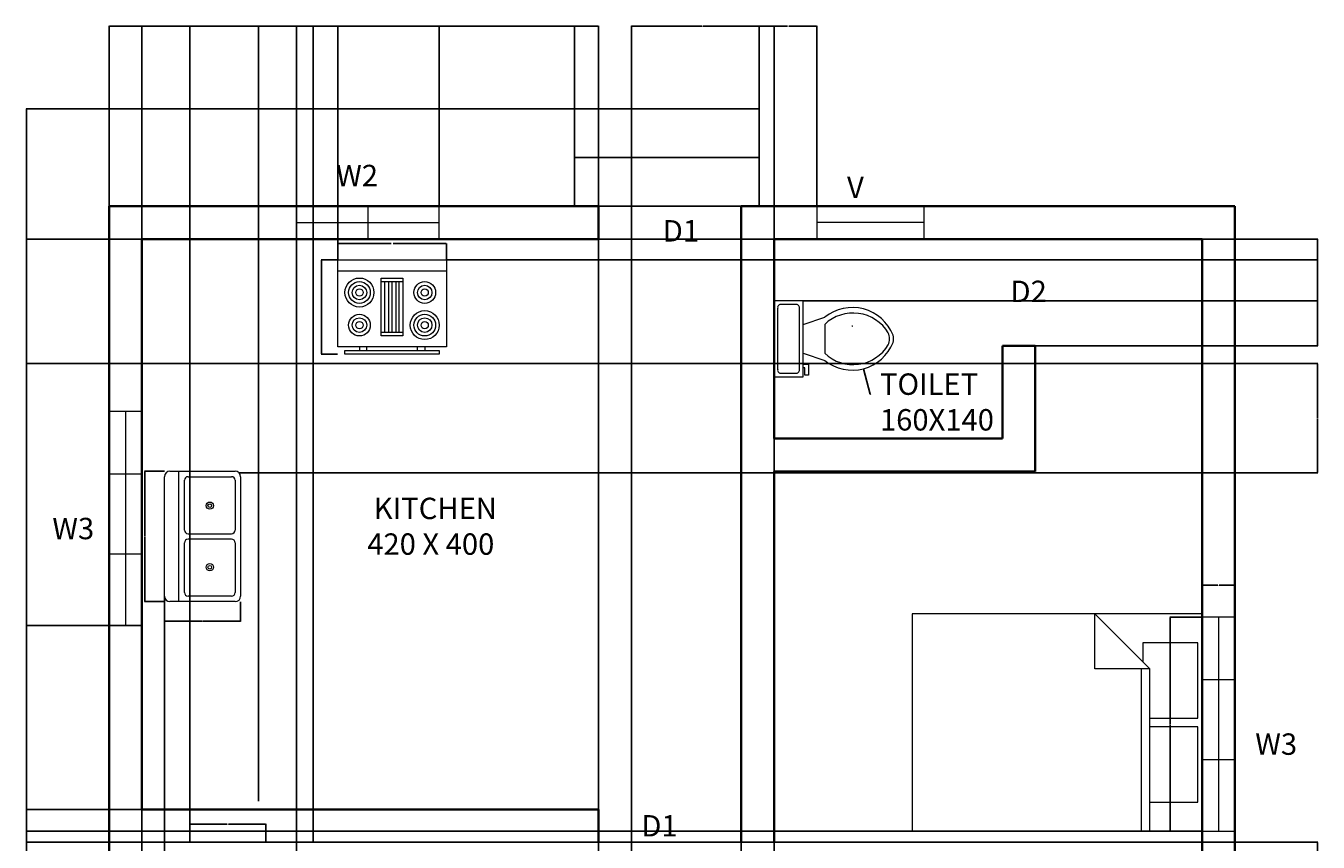
# Model space of a CAD drawing. Units: centimetres. Extents: x 575 to 1481, y 1225 to 2490.
# Tile 3 of 3: x 575 to 1481, y 1918 to 2490. Entities that reach past the tile are written whole.
import ezdxf

# ---------------------------------------------------------------- set-up
doc = ezdxf.new("R2010")
doc.units = ezdxf.units.CM
for name, color, linetype, lineweight in [('A-ANNO-DIMS', 2, 'Continuous', 18), ('A-ANNO-TEXT', 3, 'Continuous', 18), ('A-AREA-IDEN', 7, 'Continuous', 18), ('A-EQPM', 8, 'Continuous', 18), ('A-FLOR-CASE', 8, 'Continuous', 18), ('A-FLOR-FIXT', 9, 'Continuous', 18), ('A-FLOR-STRS', 7, 'Continuous', 25), ('A-FURN', 8, 'Continuous', 18), ('A-GLAZ', 4, 'Continuous', 18), ('A-WALL', 7, 'Continuous', 35)]:
    doc.layers.add(name, color=color, linetype=linetype, lineweight=lineweight)
doc.styles.get("Standard").update_dxf_attribs({"font": 'arial.ttf'})
doc.dimstyles.get("Standard").update_dxf_attribs({"dimtxt": 0.18, "dimasz": 0.18, "dimexe": 0.18, "dimexo": 0.0625, "dimgap": 0.09, "dimtad": 0, "dimtih": 1, "dimtoh": 1, "dimdec": 4, "dimzin": 0, "dimdsep": 46, "dimtxsty": 'Standard', "dimcen": 0.09, "dimadec": 0, "dimazin": 0, "dimtfac": 1, "dimtdec": 4, "dimtofl": 0, "dimtmove": 0, "dimatfit": 3, "dimfxl": 1, "dimtolj": 1, "dimtzin": 0, "dimarcsym": 0})

# ---------------------------------------------------------------- blocks, each defined once
blk = doc.blocks.new('Toilet - top')
for p, q in [((9.5, -6), (9.5, -2)), ((-10, -8.5), (-8, -8.5)), ((-10, -9.5), (-10, -8.5)), ((-7, -9.5), (-10, -9.5)), ((-8, -8.5), (-8, -8)), ((-7, -8), (-7, -9.5)), ((-4, -8), (-6, -14)), ((4, -8), (6, -14)), ((4, -14), (-4, -14))]:
    blk.add_line(p, q)
blk.add_lwpolyline([(10.5, -8), (10.5, 0), (-10.5, 0), (-10.5, -8)], close=True)
for points in [[(-9.5, -2), (-9.5, -6)], [(8.5, -1), (-8.5, -1)], [(-8.5, -7), (8.5, -7)]]:
    blk.add_lwpolyline(points)
for centre, radius, start, end in [((-8.62, -1.88), 0.884, 81.8699, 188.1301), ((8.62, -1.88), 0.884, 351.8699, 98.1301), ((-8.62, -6.12), 0.884, 171.8699, 278.1301), ((8.62, -6.12), 0.884, 261.8699, 8.1301), ((3.52, -21.58), 12.17, 141.4691, 247.9714), ((4.2, -21.82), 11.33, 136.3677, 238.9468), ((-3.52, -21.58), 12.17, 292.0284, 38.5307), ((-4.2, -21.82), 11.33, 301.053, 43.6321), ((0, -27.88), 4, 245.7318, 294.2682), ((0, -29), 4, 254.8605, 285.1395)]:
    blk.add_arc(centre, radius, start, end)
blk = doc.blocks.new('Range-Oven - 30 in top')
for p, q in [((0, -3), (30, -3)), ((12, -6), (18, -6)), ((13, -20), (13, -6)), ((14, -6), (14, -20)), ((15, -20), (15, -6)), ((16, -6), (16, -20)), ((17, -20), (17, -6)), ((18, -20), (12, -20)), ((6, -24), (6, -25)), ((8, -25), (8, -24)), ((22, -25), (22, -24)), ((24, -24), (24, -25))]:
    blk.add_line(p, q)
for points in [[(0, -24), (0, 0), (30, 0), (30, -24)], [(12, -21), (12, -5), (18, -5), (18, -21)], [(2, -26), (2, -25), (28, -25), (28, -26)]]:
    blk.add_lwpolyline(points, close=True)
for centre, radius in [((6, -9), 4), ((6, -9), 3), ((6, -9), 2), ((24, -9), 3), ((24, -9), 2), ((6, -9), 1), ((24, -9), 1), ((24, -18), 4), ((6, -18), 3), ((6, -18), 2), ((6, -18), 1), ((24, -18), 3), ((24, -18), 2), ((24, -18), 1)]:
    blk.add_circle(centre, radius)
blk = doc.blocks.new('Sink-double - 36 in top')
for p, q in [((-18, -4), (18, -4)), ((-0.75, -18.5), (-0.75, -6.5)), ((0.75, -6.5), (0.75, -18.5))]:
    blk.add_line(p, q)
for points in [[(-16.5, 0), (16.5, 0)], [(-18, -19.5), (-18, -1.5)], [(18, -1.5), (18, -19.5)], [(-16.5, -18.5), (-16.5, -6.5)], [(-15.5, -5.5), (-1.75, -5.5)], [(1.75, -5.5), (15.5, -5.5)], [(16.5, -6.5), (16.5, -18.5)], [(16.5, -21), (-16.5, -21)], [(-1.75, -19.5), (-15.5, -19.5)], [(15.5, -19.5), (1.75, -19.5)]]:
    blk.add_lwpolyline(points)
for centre, radius in [((-8.5, -12.5), 1), ((-8.5, -12.5), 0.5), ((8.5, -12.5), 1), ((8.5, -12.5), 0.5)]:
    blk.add_circle(centre, radius)
for centre, radius, start, end in [((-16.5, -1.5), 1.5, 90, 180), ((16.5, -1.5), 1.5, 0, 90), ((-15.5, -6.5), 1, 90, 180), ((-1.75, -6.5), 1, 0, 90), ((1.75, -6.5), 1, 90, 180), ((15.5, -6.5), 1, 0, 90), ((-16.5, -19.5), 1.5, 180, 270), ((-15.5, -18.5), 1, 180, 270), ((-1.75, -18.5), 1, 270, 0), ((1.75, -18.5), 1, 180, 270), ((15.5, -18.5), 1, 270, 0), ((16.5, -19.5), 1.5, 270, 0)]:
    blk.add_arc(centre, radius, start, end)
blk = doc.blocks.new('Bed - Queen')
for p, q in [((0, -80.00003), (0, 0)), ((0, 0), (59.99999, 0)), ((59.99999, 0), (59.99999, -80.00003)), ((7.99999, -1.2), (28.79998, -1.2)), ((7.99999, -14.4), (7.99999, -1.2)), ((28.79998, -1.2), (28.79998, -14.4)), ((31.19999, -1.2), (51.99999, -1.2)), ((31.19999, -14.4), (31.19999, -1.2)), ((51.99999, -1.2), (51.99999, -16.4)), ((0, -14.4), (44.8, -14.4)), ((44.8, -16.8), (0, -16.8)), ((59.99999, -29.6), (44.8, -14.4)), ((44.8, -14.4), (44.8, -29.6)), ((51.99999, -16.4), (46.79936, -16.4)), ((44.8, -29.6), (59.99999, -29.6)), ((59.99999, -80.00003), (0, -80.00003))]:
    blk.add_line(p, q)
blk = doc.blocks.new('WIN-W2-100CM')
for p, q in [((0, 0), (0, 23)), ((50, 23), (50, 0)), ((100, 0), (100, 23)), ((0, 11.5), (100, 11.5))]:
    blk.add_line(p, q)
blk = doc.blocks.new('WIN-W3-150CM')
for p, q in [((11.5, 150), (11.5, 0)), ((0, 106.3), (23, 106.3)), ((0, 50.18), (23, 50.18))]:
    blk.add_line(p, q)
blk.add_lwpolyline([(23, 0), (23, 150), (0, 150), (0, 0)], close=True)
blk = doc.blocks.new('ENTRY-STEPS')
for p, q in [((0, 0), (0, 68.38)), ((129.45, 68.38), (0, 68.38)), ((129.45, 0), (129.45, 68.38)), ((129.45, 34.19), (0, 34.19)), ((129.45, 0), (0, 0))]:
    blk.add_line(p, q)
blk = doc.blocks.new('VENT-75CM')
for p, q in [((0, 23), (0, 0)), ((75, 23), (75, 0)), ((75, 11.5), (0, 11.5))]:
    blk.add_line(p, q)
blk = doc.blocks.new('*D12')
at = {"layer": 'A-ANNO-DIMS', "color": 0, "lineweight": -2, "transparency": 16777216}
for p, q in [((1399.39, 2075.38), (1376.78, 2075.38)), ((1376.96, 2075.2), (1376.96, 2000.57)), ((1376.96, 1925.56), (1376.96, 2000.2)), ((1399.39, 1925.38), (1376.78, 1925.38))]:
    blk.add_line(p, q, dxfattribs=at)
at = {"layer": 'A-ANNO-DIMS', "color": 0, "transparency": 16777216}
for points in [[(1376.93, 2075.2), (1376.99, 2075.2), (1376.96, 2075.38)], [(1376.93, 1925.56), (1376.99, 1925.56), (1376.96, 1925.38)]]:
    blk.add_solid(points, dxfattribs=at)
at = {"layer": 'Defpoints', "color": 0, "transparency": 16777216}
for p in [(1376.96, 2075.38), (1399.46, 2075.38), (1399.46, 1925.38)]:
    blk.add_point(p, dxfattribs=at)
at = {"layer": 'A-ANNO-DIMS', "color": 0, "transparency": 16777216, "insert": (1376.96, 2000.38), "char_height": 0.18, "attachment_point": 5}
blk.add_mtext('\\A1;W3 150 TYP.', dxfattribs=at)
blk = doc.blocks.new('*D13')
at = {"layer": 'A-ANNO-DIMS', "color": 0, "lineweight": -2, "transparency": 16777216}
for p, q in [((1399.46, 2075.45), (1399.46, 2098.06)), ((1399.64, 2097.88), (1410.43, 2097.88)), ((1422.28, 2097.88), (1411.49, 2097.88)), ((1422.46, 2075.45), (1422.46, 2098.06))]:
    blk.add_line(p, q, dxfattribs=at)
at = {"layer": 'A-ANNO-DIMS', "color": 0, "transparency": 16777216}
for points in [[(1399.64, 2097.91), (1399.64, 2097.85), (1399.46, 2097.88)], [(1422.28, 2097.91), (1422.28, 2097.85), (1422.46, 2097.88)]]:
    blk.add_solid(points, dxfattribs=at)
at = {"layer": 'Defpoints', "color": 0, "transparency": 16777216}
for p in [(1422.46, 2097.88), (1399.46, 2075.38), (1422.46, 2075.38)]:
    blk.add_point(p, dxfattribs=at)
at = {"layer": 'A-ANNO-DIMS', "color": 0, "transparency": 16777216, "insert": (1410.96, 2097.88), "char_height": 0.18, "attachment_point": 5}
blk.add_mtext('\\A1;23 TYP.', dxfattribs=at)
blk = doc.blocks.new('*D21')
at = {"layer": 'A-ANNO-DIMS', "color": 0, "lineweight": -2, "transparency": 16777216}
for p, q in [((690.03, 1917.63), (690.03, 1930.34)), ((690.21, 1930.16), (716.17, 1930.16)), ((743.19, 1930.16), (717.23, 1930.16)), ((743.37, 1917.63), (743.37, 1930.34))]:
    blk.add_line(p, q, dxfattribs=at)
at = {"layer": 'A-ANNO-DIMS', "color": 0, "transparency": 16777216}
for points in [[(690.21, 1930.19), (690.21, 1930.13), (690.03, 1930.16)], [(743.19, 1930.19), (743.19, 1930.13), (743.37, 1930.16)]]:
    blk.add_solid(points, dxfattribs=at)
at = {"layer": 'Defpoints', "color": 0, "transparency": 16777216}
for p in [(743.37, 1930.16), (690.03, 1917.57), (743.37, 1917.57)]:
    blk.add_point(p, dxfattribs=at)
at = {"layer": 'A-ANNO-DIMS', "color": 0, "transparency": 16777216, "insert": (716.7, 1930.16), "char_height": 0.18, "attachment_point": 5}
blk.add_mtext('\\A1;53 TYP.', dxfattribs=at)
blk = doc.blocks.new('*D24')
at = {"layer": 'A-ANNO-DIMS', "color": 0, "lineweight": -2, "transparency": 16777216}
for p, q in [((793.68, 2325.96), (793.68, 2337.51)), ((793.86, 2337.33), (831.09, 2337.33)), ((869.7, 2337.33), (832.48, 2337.33)), ((869.88, 2325.96), (869.88, 2337.51))]:
    blk.add_line(p, q, dxfattribs=at)
at = {"layer": 'A-ANNO-DIMS', "color": 0, "transparency": 16777216}
for points in [[(793.86, 2337.36), (793.86, 2337.3), (793.68, 2337.33)], [(869.7, 2337.36), (869.7, 2337.3), (869.88, 2337.33)]]:
    blk.add_solid(points, dxfattribs=at)
at = {"layer": 'Defpoints', "color": 0, "transparency": 16777216}
for p in [(869.88, 2337.33), (793.68, 2325.9), (869.88, 2325.9)]:
    blk.add_point(p, dxfattribs=at)
at = {"layer": 'A-ANNO-DIMS', "color": 0, "transparency": 16777216, "insert": (831.78, 2337.33), "char_height": 0.18, "attachment_point": 5}
blk.add_mtext('\\A1;RANGE 76', dxfattribs=at)
blk = doc.blocks.new('*D25')
at = {"layer": 'A-ANNO-DIMS', "color": 0, "lineweight": -2, "transparency": 16777216}
for p, q in [((793.62, 2325.9), (782.07, 2325.9)), ((782.25, 2325.72), (782.25, 2293.06)), ((782.25, 2260.04), (782.25, 2292.7)), ((793.62, 2259.86), (782.07, 2259.86))]:
    blk.add_line(p, q, dxfattribs=at)
at = {"layer": 'A-ANNO-DIMS', "color": 0, "transparency": 16777216}
for points in [[(782.22, 2325.72), (782.28, 2325.72), (782.25, 2325.9)], [(782.22, 2260.04), (782.28, 2260.04), (782.25, 2259.86)]]:
    blk.add_solid(points, dxfattribs=at)
at = {"layer": 'Defpoints', "color": 0, "transparency": 16777216}
for p in [(782.25, 2325.9), (793.68, 2325.9), (793.68, 2259.86)]:
    blk.add_point(p, dxfattribs=at)
at = {"layer": 'A-ANNO-DIMS', "color": 0, "transparency": 16777216, "insert": (782.25, 2292.88), "char_height": 0.18, "attachment_point": 5}
blk.add_mtext('\\A1;66', dxfattribs=at)
blk = doc.blocks.new('*D26')
at = {"layer": 'A-ANNO-DIMS', "color": 0, "lineweight": -2, "transparency": 16777216}
for p, q in [((672.23, 2177.71), (658.4, 2177.71)), ((658.58, 2177.53), (658.58, 2132.17)), ((658.58, 2086.45), (658.58, 2131.8)), ((672.23, 2086.27), (658.4, 2086.27))]:
    blk.add_line(p, q, dxfattribs=at)
at = {"layer": 'A-ANNO-DIMS', "color": 0, "transparency": 16777216}
for points in [[(658.55, 2177.53), (658.61, 2177.53), (658.58, 2177.71)], [(658.55, 2086.45), (658.61, 2086.45), (658.58, 2086.27)]]:
    blk.add_solid(points, dxfattribs=at)
at = {"layer": 'Defpoints', "color": 0, "transparency": 16777216}
for p in [(658.58, 2177.71), (672.3, 2177.71), (672.3, 2086.27)]:
    blk.add_point(p, dxfattribs=at)
at = {"layer": 'A-ANNO-DIMS', "color": 0, "transparency": 16777216, "insert": (658.58, 2131.99), "char_height": 0.18, "attachment_point": 5}
blk.add_mtext('\\A1;SINK 91', dxfattribs=at)
blk = doc.blocks.new('*D27')
at = {"layer": 'A-ANNO-DIMS', "color": 0, "lineweight": -2, "transparency": 16777216}
for p, q in [((672.3, 2086.2), (672.3, 2072.37)), ((725.64, 2086.2), (725.64, 2072.37)), ((672.48, 2072.55), (698.75, 2072.55)), ((725.46, 2072.55), (699.19, 2072.55))]:
    blk.add_line(p, q, dxfattribs=at)
at = {"layer": 'A-ANNO-DIMS', "color": 0, "transparency": 16777216}
for points in [[(672.48, 2072.58), (672.48, 2072.52), (672.3, 2072.55)], [(725.46, 2072.58), (725.46, 2072.52), (725.64, 2072.55)]]:
    blk.add_solid(points, dxfattribs=at)
at = {"layer": 'Defpoints', "color": 0, "transparency": 16777216}
for p in [(672.3, 2086.27), (725.64, 2086.27), (672.3, 2072.55)]:
    blk.add_point(p, dxfattribs=at)
at = {"layer": 'A-ANNO-DIMS', "color": 0, "transparency": 16777216, "insert": (698.97, 2072.55), "char_height": 0.18, "attachment_point": 5}
blk.add_mtext('\\A1;53', dxfattribs=at)
blk = doc.blocks.new('*D29')
at = {"layer": 'A-ANNO-DIMS', "color": 0, "lineweight": -2, "transparency": 16777216}
for p, q in [((959.64, 2431.95), (575.33, 2431.95)), ((575.51, 2431.77), (575.51, 1857.75)), ((575.51, 1283.37), (575.51, 1857.38)), ((999.39, 1283.19), (575.33, 1283.19))]:
    blk.add_line(p, q, dxfattribs=at)
at = {"layer": 'A-ANNO-DIMS', "color": 0, "transparency": 16777216}
for points in [[(575.48, 2431.77), (575.54, 2431.77), (575.51, 2431.95)], [(575.48, 1283.37), (575.54, 1283.37), (575.51, 1283.19)]]:
    blk.add_solid(points, dxfattribs=at)
at = {"layer": 'Defpoints', "color": 0, "transparency": 16777216}
for p in [(575.51, 2431.95), (959.71, 2431.95), (999.46, 1283.19)]:
    blk.add_point(p, dxfattribs=at)
at = {"layer": 'A-ANNO-DIMS', "color": 0, "transparency": 16777216, "insert": (575.51, 1857.57), "char_height": 0.18, "attachment_point": 5}
blk.add_mtext('\\A1;1148.8', dxfattribs=at)
blk = doc.blocks.new('*D30')
at = {"layer": 'A-ANNO-DIMS', "color": 0, "lineweight": -2, "transparency": 16777216}
for p, q in [((656.46, 1374.63), (656.46, 2490.08)), ((656.64, 2489.9), (710.12, 2489.9)), ((764.52, 2489.9), (711.03, 2489.9)), ((764.7, 1374.63), (764.7, 2490.08))]:
    blk.add_line(p, q, dxfattribs=at)
at = {"layer": 'A-ANNO-DIMS', "color": 0, "transparency": 16777216}
for points in [[(656.64, 2489.93), (656.64, 2489.87), (656.46, 2489.9)], [(764.52, 2489.93), (764.52, 2489.87), (764.7, 2489.9)]]:
    blk.add_solid(points, dxfattribs=at)
at = {"layer": 'Defpoints', "color": 0, "transparency": 16777216}
for p in [(764.7, 2489.9), (656.46, 1374.57), (764.7, 1374.57)]:
    blk.add_point(p, dxfattribs=at)
at = {"layer": 'A-ANNO-DIMS', "color": 0, "transparency": 16777216, "insert": (710.58, 2489.9), "char_height": 0.18, "attachment_point": 5}
blk.add_mtext('\\A1;108.24', dxfattribs=at)
blk = doc.blocks.new('*D34')
at = {"layer": 'A-ANNO-DIMS', "color": 0, "lineweight": -2, "transparency": 16777216}
for p, q in [((656.39, 2069.5), (575.33, 2069.5)), ((575.51, 2069.32), (575.51, 2005.21)), ((575.51, 1940.75), (575.51, 2004.85)), ((656.39, 1940.57), (575.33, 1940.57))]:
    blk.add_line(p, q, dxfattribs=at)
at = {"layer": 'A-ANNO-DIMS', "color": 0, "transparency": 16777216}
for points in [[(575.48, 2069.32), (575.54, 2069.32), (575.51, 2069.5)], [(575.48, 1940.75), (575.54, 1940.75), (575.51, 1940.57)]]:
    blk.add_solid(points, dxfattribs=at)
at = {"layer": 'Defpoints', "color": 0, "transparency": 16777216}
for p in [(575.51, 2069.5), (656.46, 2069.5), (656.46, 1940.57)]:
    blk.add_point(p, dxfattribs=at)
at = {"layer": 'A-ANNO-DIMS', "color": 0, "transparency": 16777216, "insert": (575.51, 2005.03), "char_height": 0.18, "attachment_point": 5}
blk.add_mtext('\\A1;128.93', dxfattribs=at)
blk = doc.blocks.new('*D35')
at = {"layer": 'A-ANNO-DIMS', "color": 0, "lineweight": -2, "transparency": 16777216}
for p, q in [((633.46, 2363.63), (633.46, 2490.08)), ((633.64, 2489.9), (698.62, 2489.9)), ((764.52, 2489.9), (699.53, 2489.9)), ((764.7, 2363.63), (764.7, 2490.08))]:
    blk.add_line(p, q, dxfattribs=at)
at = {"layer": 'A-ANNO-DIMS', "color": 0, "transparency": 16777216}
for points in [[(633.64, 2489.93), (633.64, 2489.87), (633.46, 2489.9)], [(764.52, 2489.93), (764.52, 2489.87), (764.7, 2489.9)]]:
    blk.add_solid(points, dxfattribs=at)
at = {"layer": 'Defpoints', "color": 0, "transparency": 16777216}
for p in [(764.7, 2489.9), (633.46, 2363.57), (764.7, 2363.57)]:
    blk.add_point(p, dxfattribs=at)
at = {"layer": 'A-ANNO-DIMS', "color": 0, "transparency": 16777216, "insert": (699.08, 2489.9), "char_height": 0.18, "attachment_point": 5}
blk.add_mtext('\\A1;131.24', dxfattribs=at)
blk = doc.blocks.new('*D36')
at = {"layer": 'A-ANNO-DIMS', "color": 0, "lineweight": -2, "transparency": 16777216}
for p, q in [((864.7, 2363.63), (864.7, 2490.08)), ((864.88, 2489.9), (911.98, 2489.9)), ((959.53, 2489.9), (912.42, 2489.9)), ((959.71, 2363.63), (959.71, 2490.08))]:
    blk.add_line(p, q, dxfattribs=at)
at = {"layer": 'A-ANNO-DIMS', "color": 0, "transparency": 16777216}
for points in [[(864.88, 2489.93), (864.88, 2489.87), (864.7, 2489.9)], [(959.53, 2489.93), (959.53, 2489.87), (959.71, 2489.9)]]:
    blk.add_solid(points, dxfattribs=at)
at = {"layer": 'Defpoints', "color": 0, "transparency": 16777216}
for p in [(959.71, 2489.9), (864.7, 2363.57), (959.71, 2363.57)]:
    blk.add_point(p, dxfattribs=at)
at = {"layer": 'A-ANNO-DIMS', "color": 0, "transparency": 16777216, "insert": (912.2, 2489.9), "char_height": 0.18, "attachment_point": 5}
blk.add_mtext('\\A1;95', dxfattribs=at)
blk = doc.blocks.new('*D37')
at = {"layer": 'A-ANNO-DIMS', "color": 0, "lineweight": -2, "transparency": 16777216}
for p, q in [((1076.46, 2363.5), (1076.46, 1225.06)), ((976.46, 2340.5), (976.46, 1225.06)), ((976.64, 1225.24), (1026.18, 1225.24)), ((1076.28, 1225.24), (1026.74, 1225.24))]:
    blk.add_line(p, q, dxfattribs=at)
at = {"layer": 'A-ANNO-DIMS', "color": 0, "transparency": 16777216}
for points in [[(976.64, 1225.27), (976.64, 1225.21), (976.46, 1225.24)], [(1076.28, 1225.27), (1076.28, 1225.21), (1076.46, 1225.24)]]:
    blk.add_solid(points, dxfattribs=at)
at = {"layer": 'Defpoints', "color": 0, "transparency": 16777216}
for p in [(1076.46, 2363.57), (976.46, 2340.57), (1076.46, 1225.24)]:
    blk.add_point(p, dxfattribs=at)
at = {"layer": 'A-ANNO-DIMS', "color": 0, "transparency": 16777216, "insert": (1026.46, 1225.24), "char_height": 0.18, "attachment_point": 5}
blk.add_mtext('\\A1;100', dxfattribs=at)
blk = doc.blocks.new('*D38')
at = {"layer": 'A-ANNO-DIMS', "color": 0, "lineweight": -2, "transparency": 16777216}
for p, q in [((1089.15, 2363.63), (1089.15, 2490.08)), ((1089.33, 2489.9), (1108.93, 2489.9)), ((1129.33, 2489.9), (1109.73, 2489.9)), ((1129.51, 2363.63), (1129.51, 2490.08))]:
    blk.add_line(p, q, dxfattribs=at)
at = {"layer": 'A-ANNO-DIMS', "color": 0, "transparency": 16777216}
for points in [[(1089.33, 2489.93), (1089.33, 2489.87), (1089.15, 2489.9)], [(1129.33, 2489.93), (1129.33, 2489.87), (1129.51, 2489.9)]]:
    blk.add_solid(points, dxfattribs=at)
at = {"layer": 'Defpoints', "color": 0, "transparency": 16777216}
for p in [(1129.51, 2489.9), (1089.15, 2363.57), (1129.51, 2363.57)]:
    blk.add_point(p, dxfattribs=at)
at = {"layer": 'A-ANNO-DIMS', "color": 0, "transparency": 16777216, "insert": (1109.33, 2489.9), "char_height": 0.18, "attachment_point": 5}
blk.add_mtext('\\A1;40.35', dxfattribs=at)
blk = doc.blocks.new('*D40')
at = {"layer": 'A-ANNO-DIMS', "color": 0, "lineweight": -2, "transparency": 16777216}
for p, q in [((1399.39, 1925.38), (575.33, 1925.38)), ((575.51, 1925.2), (575.51, 1881.66)), ((575.51, 1837.75), (575.51, 1881.29)), ((1399.39, 1837.57), (575.33, 1837.57))]:
    blk.add_line(p, q, dxfattribs=at)
at = {"layer": 'A-ANNO-DIMS', "color": 0, "transparency": 16777216}
for points in [[(575.48, 1925.2), (575.54, 1925.2), (575.51, 1925.38)], [(575.48, 1837.75), (575.54, 1837.75), (575.51, 1837.57)]]:
    blk.add_solid(points, dxfattribs=at)
at = {"layer": 'Defpoints', "color": 0, "transparency": 16777216}
for p in [(575.51, 1925.38), (1399.46, 1925.38), (1399.46, 1837.57)]:
    blk.add_point(p, dxfattribs=at)
at = {"layer": 'A-ANNO-DIMS', "color": 0, "transparency": 16777216, "insert": (575.51, 1881.47), "char_height": 0.18, "attachment_point": 5}
blk.add_mtext('\\A1;87.82', dxfattribs=at)
blk = doc.blocks.new('*D41')
at = {"layer": 'A-ANNO-DIMS', "color": 0, "lineweight": -2, "transparency": 16777216}
for p, q in [((776.46, 1917.63), (776.46, 2490.08)), ((776.64, 2489.9), (876.17, 2489.9)), ((976.28, 2489.9), (876.75, 2489.9)), ((976.46, 1917.63), (976.46, 2490.08))]:
    blk.add_line(p, q, dxfattribs=at)
at = {"layer": 'A-ANNO-DIMS', "color": 0, "transparency": 16777216}
for points in [[(776.64, 2489.93), (776.64, 2489.87), (776.46, 2489.9)], [(976.28, 2489.93), (976.28, 2489.87), (976.46, 2489.9)]]:
    blk.add_solid(points, dxfattribs=at)
at = {"layer": 'Defpoints', "color": 0, "transparency": 16777216}
for p in [(976.46, 2489.9), (776.46, 1917.57), (976.46, 1917.57)]:
    blk.add_point(p, dxfattribs=at)
at = {"layer": 'A-ANNO-DIMS', "color": 0, "transparency": 16777216, "insert": (876.46, 2489.9), "char_height": 0.18, "attachment_point": 5}
blk.add_mtext('\\A1;200', dxfattribs=at)
blk = doc.blocks.new('*D42')
at = {"layer": 'A-ANNO-DIMS', "color": 0, "lineweight": -2, "transparency": 16777216}
for p, q in [((976.52, 1917.57), (1480.59, 1917.57)), ((1480.41, 1917.39), (1480.41, 1867.75)), ((1480.41, 1817.75), (1480.41, 1867.38)), ((976.52, 1817.57), (1480.59, 1817.57))]:
    blk.add_line(p, q, dxfattribs=at)
at = {"layer": 'A-ANNO-DIMS', "color": 0, "transparency": 16777216}
for points in [[(1480.38, 1917.39), (1480.44, 1917.39), (1480.41, 1917.57)], [(1480.38, 1817.75), (1480.44, 1817.75), (1480.41, 1817.57)]]:
    blk.add_solid(points, dxfattribs=at)
at = {"layer": 'Defpoints', "color": 0, "transparency": 16777216}
for p in [(976.46, 1917.57), (1480.41, 1917.57), (976.46, 1817.57)]:
    blk.add_point(p, dxfattribs=at)
at = {"layer": 'A-ANNO-DIMS', "color": 0, "transparency": 16777216, "insert": (1480.41, 1867.57), "char_height": 0.18, "attachment_point": 5}
blk.add_mtext('\\A1;100', dxfattribs=at)
blk = doc.blocks.new('*D46')
at = {"layer": 'A-ANNO-DIMS', "color": 0, "lineweight": -2, "transparency": 16777216}
for p, q in [((1076.39, 1917.57), (575.33, 1917.57)), ((575.51, 1917.39), (575.51, 1877.75)), ((575.51, 1837.75), (575.51, 1877.38)), ((1076.39, 1837.57), (575.33, 1837.57))]:
    blk.add_line(p, q, dxfattribs=at)
at = {"layer": 'A-ANNO-DIMS', "color": 0, "transparency": 16777216}
for points in [[(575.48, 1917.39), (575.54, 1917.39), (575.51, 1917.57)], [(575.48, 1837.75), (575.54, 1837.75), (575.51, 1837.57)]]:
    blk.add_solid(points, dxfattribs=at)
at = {"layer": 'Defpoints', "color": 0, "transparency": 16777216}
for p in [(575.51, 1917.57), (1076.46, 1917.57), (1076.46, 1837.57)]:
    blk.add_point(p, dxfattribs=at)
at = {"layer": 'A-ANNO-DIMS', "color": 0, "transparency": 16777216, "insert": (575.51, 1877.57), "char_height": 0.18, "attachment_point": 5}
blk.add_mtext('\\A1;80', dxfattribs=at)
blk = doc.blocks.new('*D47')
at = {"layer": 'A-ANNO-DIMS', "color": 0, "lineweight": -2, "transparency": 16777216}
for p, q in [((1399.52, 2340.57), (1480.59, 2340.57)), ((1480.41, 2340.39), (1480.41, 2303.25)), ((1480.41, 2265.75), (1480.41, 2302.88)), ((1282.52, 2265.57), (1480.59, 2265.57))]:
    blk.add_line(p, q, dxfattribs=at)
at = {"layer": 'A-ANNO-DIMS', "color": 0, "transparency": 16777216}
for points in [[(1480.38, 2340.39), (1480.44, 2340.39), (1480.41, 2340.57)], [(1480.38, 2265.75), (1480.44, 2265.75), (1480.41, 2265.57)]]:
    blk.add_solid(points, dxfattribs=at)
at = {"layer": 'Defpoints', "color": 0, "transparency": 16777216}
for p in [(1399.46, 2340.57), (1480.41, 2340.57), (1282.46, 2265.57)]:
    blk.add_point(p, dxfattribs=at)
at = {"layer": 'A-ANNO-DIMS', "color": 0, "transparency": 16777216, "insert": (1480.41, 2303.07), "char_height": 0.18, "attachment_point": 5}
blk.add_mtext('\\A1;75', dxfattribs=at)
blk = doc.blocks.new('*D48')
at = {"layer": 'A-ANNO-DIMS', "color": 0, "lineweight": -2, "transparency": 16777216}
for p, q in [((999.46, 1351.63), (999.46, 2490.08)), ((999.64, 2489.9), (1049.18, 2489.9)), ((1099.28, 2489.9), (1049.74, 2489.9)), ((1099.46, 1451.63), (1099.46, 2490.08))]:
    blk.add_line(p, q, dxfattribs=at)
at = {"layer": 'A-ANNO-DIMS', "color": 0, "transparency": 16777216}
for points in [[(999.64, 2489.93), (999.64, 2489.87), (999.46, 2489.9)], [(1099.28, 2489.93), (1099.28, 2489.87), (1099.46, 2489.9)]]:
    blk.add_solid(points, dxfattribs=at)
at = {"layer": 'Defpoints', "color": 0, "transparency": 16777216}
for p in [(1099.46, 2489.9), (1099.46, 1451.57), (999.46, 1351.57)]:
    blk.add_point(p, dxfattribs=at)
at = {"layer": 'A-ANNO-DIMS', "color": 0, "transparency": 16777216, "insert": (1049.46, 2489.9), "char_height": 0.18, "attachment_point": 5}
blk.add_mtext('\\A1;100', dxfattribs=at)
blk = doc.blocks.new('*D49')
at = {"layer": 'A-ANNO-DIMS', "color": 0, "lineweight": -2, "transparency": 16777216}
for p, q in [((656.46, 1940.63), (656.46, 2490.08)), ((656.64, 2489.9), (696.94, 2489.9)), ((738.03, 2489.9), (697.73, 2489.9)), ((738.21, 1946.28), (738.21, 2490.08))]:
    blk.add_line(p, q, dxfattribs=at)
at = {"layer": 'A-ANNO-DIMS', "color": 0, "transparency": 16777216}
for points in [[(656.64, 2489.93), (656.64, 2489.87), (656.46, 2489.9)], [(738.03, 2489.93), (738.03, 2489.87), (738.21, 2489.9)]]:
    blk.add_solid(points, dxfattribs=at)
at = {"layer": 'Defpoints', "color": 0, "transparency": 16777216}
for p in [(738.21, 2489.9), (656.46, 1940.57), (738.21, 1946.22)]:
    blk.add_point(p, dxfattribs=at)
at = {"layer": 'A-ANNO-DIMS', "color": 0, "transparency": 16777216, "insert": (697.33, 2489.9), "char_height": 0.18, "attachment_point": 5}
blk.add_mtext('\\A1;81.75', dxfattribs=at)
blk = doc.blocks.new('*D50')
at = {"layer": 'A-ANNO-DIMS', "color": 0, "lineweight": -2, "transparency": 16777216}
for p, q in [((764.64, 2340.57), (575.33, 2340.57)), ((575.51, 2340.39), (575.51, 2297.06)), ((575.51, 2253.38), (575.51, 2296.7)), ((738.14, 2253.2), (575.33, 2253.2))]:
    blk.add_line(p, q, dxfattribs=at)
at = {"layer": 'A-ANNO-DIMS', "color": 0, "transparency": 16777216}
for points in [[(575.48, 2340.39), (575.54, 2340.39), (575.51, 2340.57)], [(575.48, 2253.38), (575.54, 2253.38), (575.51, 2253.2)]]:
    blk.add_solid(points, dxfattribs=at)
at = {"layer": 'Defpoints', "color": 0, "transparency": 16777216}
for p in [(575.51, 2340.57), (764.7, 2340.57), (738.21, 2253.2)]:
    blk.add_point(p, dxfattribs=at)
at = {"layer": 'A-ANNO-DIMS', "color": 0, "transparency": 16777216, "insert": (575.51, 2296.88), "char_height": 0.18, "attachment_point": 5}
blk.add_mtext('\\A1;87.37', dxfattribs=at)
blk = doc.blocks.new('*D51')
at = {"layer": 'A-ANNO-DIMS', "color": 0, "lineweight": -2, "transparency": 16777216}
for p, q in [((656.46, 2340.63), (656.46, 2490.08)), ((656.64, 2489.9), (724.62, 2489.9)), ((793.5, 2489.9), (725.53, 2489.9)), ((793.68, 2325.96), (793.68, 2490.08))]:
    blk.add_line(p, q, dxfattribs=at)
at = {"layer": 'A-ANNO-DIMS', "color": 0, "transparency": 16777216}
for points in [[(656.64, 2489.93), (656.64, 2489.87), (656.46, 2489.9)], [(793.5, 2489.93), (793.5, 2489.87), (793.68, 2489.9)]]:
    blk.add_solid(points, dxfattribs=at)
at = {"layer": 'Defpoints', "color": 0, "transparency": 16777216}
for p in [(793.68, 2489.9), (656.46, 2340.57), (793.68, 2325.9)]:
    blk.add_point(p, dxfattribs=at)
at = {"layer": 'A-ANNO-DIMS', "color": 0, "transparency": 16777216, "insert": (725.07, 2489.9), "char_height": 0.18, "attachment_point": 5}
blk.add_mtext('\\A1;137.23', dxfattribs=at)
blk = doc.blocks.new('*D52')
at = {"layer": 'A-ANNO-DIMS', "color": 0, "lineweight": -2, "transparency": 16777216}
for p, q in [((738.27, 2253.2), (1480.59, 2253.2)), ((1480.41, 2253.02), (1480.41, 2215.07)), ((1480.41, 2176.77), (1480.41, 2214.71)), ((724.58, 2176.59), (1480.59, 2176.59))]:
    blk.add_line(p, q, dxfattribs=at)
at = {"layer": 'A-ANNO-DIMS', "color": 0, "transparency": 16777216}
for points in [[(1480.38, 2253.02), (1480.44, 2253.02), (1480.41, 2253.2)], [(1480.38, 2176.77), (1480.44, 2176.77), (1480.41, 2176.59)]]:
    blk.add_solid(points, dxfattribs=at)
at = {"layer": 'Defpoints', "color": 0, "transparency": 16777216}
for p in [(738.21, 2253.2), (724.52, 2176.59), (1480.41, 2176.59)]:
    blk.add_point(p, dxfattribs=at)
at = {"layer": 'A-ANNO-DIMS', "color": 0, "transparency": 16777216, "insert": (1480.41, 2214.89), "char_height": 0.18, "attachment_point": 5}
blk.add_mtext('\\A1;76.6', dxfattribs=at)
blk = doc.blocks.new('*D53')
at = {"layer": 'A-ANNO-DIMS', "color": 0, "lineweight": -2, "transparency": 16777216}
for p, q in [((864.76, 2340.57), (1480.59, 2340.57)), ((1480.41, 2340.39), (1480.41, 2333.42)), ((1480.41, 2326.08), (1480.41, 2333.05)), ((869.95, 2325.9), (1480.59, 2325.9))]:
    blk.add_line(p, q, dxfattribs=at)
at = {"layer": 'A-ANNO-DIMS', "color": 0, "transparency": 16777216}
for points in [[(1480.38, 2340.39), (1480.44, 2340.39), (1480.41, 2340.57)], [(1480.38, 2326.08), (1480.44, 2326.08), (1480.41, 2325.9)]]:
    blk.add_solid(points, dxfattribs=at)
at = {"layer": 'Defpoints', "color": 0, "transparency": 16777216}
for p in [(864.7, 2340.57), (1480.41, 2340.57), (869.88, 2325.9)]:
    blk.add_point(p, dxfattribs=at)
at = {"layer": 'A-ANNO-DIMS', "color": 0, "transparency": 16777216, "insert": (1480.41, 2333.23), "char_height": 0.18, "attachment_point": 5}
blk.add_mtext('\\A1;14.665', dxfattribs=at)
blk = doc.blocks.new('*D54')
at = {"layer": 'A-ANNO-DIMS', "color": 0, "lineweight": -2, "transparency": 16777216}
for p, q in [((656.46, 2119.61), (656.46, 1225.06)), ((672.3, 2090.01), (672.3, 1225.06)), ((656.64, 1225.24), (663.99, 1225.24)), ((672.12, 1225.24), (664.76, 1225.24))]:
    blk.add_line(p, q, dxfattribs=at)
at = {"layer": 'A-ANNO-DIMS', "color": 0, "transparency": 16777216}
for points in [[(656.64, 1225.27), (656.64, 1225.21), (656.46, 1225.24)], [(672.12, 1225.27), (672.12, 1225.21), (672.3, 1225.24)]]:
    blk.add_solid(points, dxfattribs=at)
at = {"layer": 'Defpoints', "color": 0, "transparency": 16777216}
for p in [(656.46, 2119.68), (672.3, 2090.08), (672.3, 1225.24)]:
    blk.add_point(p, dxfattribs=at)
at = {"layer": 'A-ANNO-DIMS', "color": 0, "transparency": 16777216, "insert": (664.38, 1225.24), "char_height": 0.18, "attachment_point": 5}
blk.add_mtext('\\A1;15.84', dxfattribs=at)
blk = doc.blocks.new('*D58')
at = {"layer": 'A-ANNO-DIMS', "color": 0, "lineweight": -2, "transparency": 16777216}
for p, q in [((656.46, 1917.63), (656.46, 2490.08)), ((656.64, 2489.9), (672.85, 2489.9)), ((689.85, 2489.9), (673.64, 2489.9)), ((690.03, 1917.63), (690.03, 2490.08))]:
    blk.add_line(p, q, dxfattribs=at)
at = {"layer": 'A-ANNO-DIMS', "color": 0, "transparency": 16777216}
for points in [[(656.64, 2489.93), (656.64, 2489.87), (656.46, 2489.9)], [(689.85, 2489.93), (689.85, 2489.87), (690.03, 2489.9)]]:
    blk.add_solid(points, dxfattribs=at)
at = {"layer": 'Defpoints', "color": 0, "transparency": 16777216}
for p in [(690.03, 2489.9), (656.46, 1917.57), (690.03, 1917.57)]:
    blk.add_point(p, dxfattribs=at)
at = {"layer": 'A-ANNO-DIMS', "color": 0, "transparency": 16777216, "insert": (673.24, 2489.9), "char_height": 0.18, "attachment_point": 5}
blk.add_mtext('\\A1;33.57', dxfattribs=at)
blk = doc.blocks.new('*D59')
at = {"layer": 'A-ANNO-DIMS', "color": 0, "lineweight": -2, "transparency": 16777216}
for p, q in [((1129.57, 2340.57), (1480.59, 2340.57)), ((1480.41, 2340.39), (1480.41, 2319.08)), ((1480.41, 2297.42), (1480.41, 2318.72)), ((1119.84, 2297.24), (1480.59, 2297.24))]:
    blk.add_line(p, q, dxfattribs=at)
at = {"layer": 'A-ANNO-DIMS', "color": 0, "transparency": 16777216}
for points in [[(1480.38, 2340.39), (1480.44, 2340.39), (1480.41, 2340.57)], [(1480.38, 2297.42), (1480.44, 2297.42), (1480.41, 2297.24)]]:
    blk.add_solid(points, dxfattribs=at)
at = {"layer": 'Defpoints', "color": 0, "transparency": 16777216}
for p in [(1129.51, 2340.57), (1119.78, 2297.24), (1480.41, 2297.24)]:
    blk.add_point(p, dxfattribs=at)
at = {"layer": 'A-ANNO-DIMS', "color": 0, "transparency": 16777216, "insert": (1480.41, 2318.9), "char_height": 0.18, "attachment_point": 5}
blk.add_mtext('\\A1;43.33', dxfattribs=at)
blk = doc.blocks.new('*D60')
at = {"layer": 'A-ANNO-DIMS', "color": 0, "lineweight": -2, "transparency": 16777216}
for p, q in [((1154.18, 2279.51), (1154.36, 2279.51)), ((1154.27, 2279.42), (1154.27, 2279.6)), ((1166.84, 2231.67), (1162.17, 2249.44)), ((1167.02, 2231.67), (1166.84, 2231.67))]:
    blk.add_line(p, q, dxfattribs=at)
at = {"layer": 'A-ANNO-DIMS', "color": 0, "transparency": 16777216}
blk.add_solid([(1162.2, 2249.44), (1162.14, 2249.43), (1162.13, 2249.61)], dxfattribs=at)
at = {"layer": 'Defpoints', "color": 0, "transparency": 16777216}
for p in [(1154.27, 2279.51), (1162.13, 2249.61)]:
    blk.add_point(p, dxfattribs=at)
at = {"layer": 'A-ANNO-DIMS', "color": 0, "transparency": 16777216, "insert": (1167.68, 2231.67), "char_height": 0.18, "attachment_point": 5}
blk.add_mtext('\\A1;4X R30.91', dxfattribs=at)

msp = doc.modelspace()

# ---------------------------------------------------------------- linework, layer by layer
at = {"layer": 'A-FLOR-CASE'}
for p, q in [((976.457, 2340.566), (976.457, 2253.1956)), ((738.2059, 1946.217), (738.2059, 2253.1956)), ((738.2059, 2253.1956), (976.457, 2253.1956))]:
    msp.add_line(p, q, dxfattribs=at)
at = {"layer": 'A-WALL'}
for p, q in [((633.457, 2363.566), (976.457, 2363.566)), ((633.457, 2363.566), (633.457, 1351.566)), ((976.457, 2363.566), (976.457, 2340.566)), ((1076.457, 2363.566), (1076.457, 1917.566)), ((1076.457, 2363.566), (1422.457, 2363.566)), ((1422.457, 2363.566), (1422.457, 1351.566)), ((656.457, 2340.566), (656.457, 1940.566)), ((656.457, 2340.566), (976.457, 2340.566)), ((1099.457, 2340.566), (1099.457, 2200.566)), ((1099.457, 2340.566), (1399.457, 2340.566)), ((1399.457, 2340.566), (1399.457, 1837.566)), ((1259.457, 2265.566), (1259.457, 2200.566)), ((1259.457, 2265.566), (1282.457, 2265.566)), ((1282.457, 2265.566), (1282.457, 2177.566)), ((1099.457, 2200.566), (1259.457, 2200.566)), ((1099.457, 2177.566), (1282.457, 2177.566)), ((1099.457, 2177.566), (1099.457, 1917.566)), ((656.457, 1940.566), (976.457, 1940.566)), ((976.457, 1940.566), (976.457, 1917.566))]:
    msp.add_line(p, q, dxfattribs=at)

# ---------------------------------------------------------------- block references
at = {"layer": 'A-EQPM', "xscale": 2.54, "yscale": 2.54, "zscale": 2.54}
msp.add_blockref('Range-Oven - 30 in top', (793.6846, 2325.901), dxfattribs=at)
at = {"layer": 'A-FLOR-FIXT', "xscale": 2.54, "yscale": 2.54, "zscale": 2.54, "rotation": 90}
for name, p in [('Toilet - top', (1099.457, 2270.566)), ('Sink-double - 36 in top', (672.2969, 2131.9853))]:
    msp.add_blockref(name, p, dxfattribs=at)
at = {"layer": 'A-FLOR-STRS'}
msp.add_blockref('ENTRY-STEPS', (959.705, 2363.566), dxfattribs=at)
at = {"layer": 'A-FURN', "xscale": -2.54, "yscale": 2.54, "zscale": 2.54, "rotation": 270}
msp.add_blockref('Bed - Queen', (1399.457, 1925.3838), dxfattribs=at)
at = {"layer": 'A-GLAZ'}
for name, p in [('WIN-W2-100CM', (764.7005, 2340.566)), ('VENT-75CM', (1129.507, 2340.566)), ('WIN-W3-150CM', (633.457, 2069.496)), ('WIN-W3-150CM', (1399.457, 1925.3836))]:
    msp.add_blockref(name, p, dxfattribs=at)

# ---------------------------------------------------------------- texts
at = {"layer": 'A-ANNO-TEXT', "char_height": 15, "attachment_point": 1}
for s, insert in [('W2', (792.6132, 2392.5894)), ('V', (1150.6108, 2384.2831)), ('D1', (1021.4889, 2353.7974)), ('D2', (1265.1995, 2311.3452)), ('W3', (593.6859, 2145.0187)), ('W3', (1436.7099, 1993.8298)), ('D1', (1006.4604, 1936.5523))]:
    msp.add_mtext_dynamic_manual_height_columns(s, width=230.89075, gutter_width=12.5, heights=[0], dxfattribs=dict(at, insert=insert))
at = {"layer": 'A-AREA-IDEN', "char_height": 15, "attachment_point": 1}
for s, insert in [('TOILET\\P160X140', (1173.6953, 2246.275)), ('  KITCHEN\\P 420 X 400', (809.8049, 2159.1245))]:
    msp.add_mtext_dynamic_manual_height_columns(s, width=230.89075, gutter_width=12.5, heights=[0], dxfattribs=dict(at, insert=insert))

# ---------------------------------------------------------------- dimensions: what is measured, and where the dimension line sits
at = {"layer": 'A-ANNO-DIMS'}
for base, p1, p2, override, picture, middle in [((764.7001, 2489.8956), (633.457, 2363.566), (764.7001, 2363.566), {"dimdec": 2, "dimlfac": 1, "dimrnd": 0, "dimzin": 0, "dimdsep": 46, "dimlunit": 2}, '*D35', (699.0785, 2489.8956)), ((764.7001, 2489.8956), (656.457, 1374.566), (764.7001, 1374.566), {"dimdec": 2, "dimlfac": 1, "dimrnd": 0, "dimzin": 0, "dimdsep": 46, "dimlunit": 2}, '*D30', (710.5785, 2489.8956)), ((738.2059, 2489.8956), (656.457, 1940.566), (738.2059, 1946.217), {"dimdec": 2, "dimlfac": 1, "dimrnd": 0, "dimzin": 0, "dimdsep": 46, "dimlunit": 2}, '*D49', (697.3314, 2489.8956)), ((793.6846, 2489.8956), (656.457, 2340.566), (793.6846, 2325.901), {"dimdec": 2, "dimlfac": 1, "dimrnd": 0, "dimzin": 0, "dimdsep": 46, "dimlunit": 2}, '*D51', (725.0708, 2489.8956)), ((690.0295, 2489.8956), (656.457, 1917.566), (690.0295, 1917.566), {"dimdec": 2, "dimlfac": 1, "dimrnd": 0, "dimzin": 0, "dimdsep": 46, "dimlunit": 2}, '*D58', (673.2432, 2489.8956)), ((976.457, 2489.8956), (776.457, 1917.566), (976.457, 1917.566), {"dimdec": 0, "dimlfac": 1, "dimrnd": 0, "dimzin": 0, "dimdsep": 46, "dimlunit": 2}, '*D41', (876.457, 2489.8956)), ((959.7054, 2489.8956), (864.7001, 2363.566), (959.7054, 2363.566), {"dimdec": 0, "dimlfac": 1, "dimrnd": 0, "dimzin": 0, "dimdsep": 46, "dimlunit": 2}, '*D36', (912.2027, 2489.8956)), ((1099.457, 2489.8956), (999.457, 1351.566), (1099.457, 1451.566), {"dimdec": 0, "dimlfac": 1, "dimrnd": 0, "dimzin": 0, "dimdsep": 46, "dimlunit": 2}, '*D48', (1049.457, 2489.8956)), ((1129.5074, 2489.8956), (1089.1538, 2363.566), (1129.5074, 2363.566), {"dimdec": 2, "dimlfac": 1, "dimrnd": 0, "dimzin": 0, "dimdsep": 46, "dimlunit": 2}, '*D38', (1109.3306, 2489.8956)), ((1076.457, 1225.2364), (976.457, 2340.566), (1076.457, 2363.566), {"dimdec": 0, "dimlfac": 1, "dimrnd": 0, "dimzin": 0, "dimdsep": 46, "dimlunit": 2}, '*D37', (1026.457, 1225.2364)), ((672.2969, 1225.2364), (656.457, 2119.6752), (672.2969, 2090.0753), {"dimdec": 2, "dimlfac": 1, "dimrnd": 0, "dimzin": 0, "dimdsep": 46, "dimlunit": 2}, '*D54', (664.3769, 1225.2364))]:
    dim = msp.add_linear_dim(base=base, p1=p1, p2=p2, dimstyle='Standard', override=override, dxfattribs=at)
    dim.commit()
    dim.dimension.update_dxf_attribs({"geometry": picture, "text_midpoint": middle})
for base, p1, p2, angle, override, picture, middle in [((575.507, 2431.9456), (999.457, 1283.1864), (959.7054, 2431.9456), 90, {"dimdec": 1, "dimlfac": 1, "dimrnd": 0, "dimzin": 0, "dimdsep": 46, "dimlunit": 2}, '*D29', (575.507, 1857.566)), ((575.507, 2340.566), (738.2059, 2253.1956), (764.7001, 2340.566), 90, {"dimdec": 2, "dimlfac": 1, "dimrnd": 0, "dimzin": 0, "dimdsep": 46, "dimlunit": 2}, '*D50', (575.507, 2296.8808)), ((1480.407, 2340.566), (869.8846, 2325.901), (864.7001, 2340.566), 90, {"dimdec": 3, "dimlfac": 1, "dimrnd": 0, "dimzin": 0, "dimdsep": 46, "dimlunit": 2}, '*D53', (1480.407, 2333.2335)), ((1480.407, 2297.236), (1129.5074, 2340.566), (1119.777, 2297.236), 90, {"dimdec": 2, "dimlfac": 1, "dimrnd": 0, "dimzin": 0, "dimdsep": 46, "dimlunit": 2}, '*D59', (1480.407, 2318.901)), ((1480.407, 2340.566), (1282.457, 2265.566), (1399.457, 2340.566), 90, {"dimdec": 0, "dimlfac": 1, "dimrnd": 0, "dimzin": 0, "dimdsep": 46, "dimlunit": 2}, '*D47', (1480.407, 2303.066)), ((782.2546, 2325.901), (793.6846, 2259.8611), (793.6846, 2325.901), 90, {"dimdec": 0, "dimlfac": 1, "dimrnd": 0, "dimzin": 0, "dimdsep": 46, "dimlunit": 2}, '*D25', (782.2546, 2292.881)), ((1480.407, 2176.5894), (738.2059, 2253.1956), (724.5209, 2176.5894), 90, {"dimdec": 1, "dimlfac": 1, "dimrnd": 0, "dimzin": 0, "dimdsep": 46, "dimlunit": 2}, '*D52', (1480.407, 2214.8925)), ((672.2969, 2072.5493), (725.6369, 2086.2653), (672.2969, 2086.2653), 180, {"dimdec": 0, "dimlfac": 1, "dimrnd": 0, "dimzin": 0, "dimdsep": 46, "dimlunit": 2}, '*D27', (698.9669, 2072.5493)), ((575.507, 2069.4963), (656.457, 1940.566), (656.457, 2069.4963), 90, {"dimdec": 2, "dimlfac": 1, "dimrnd": 0, "dimzin": 0, "dimdsep": 46, "dimlunit": 2}, '*D34', (575.507, 2005.0311)), ((575.507, 1925.3838), (1399.457, 1837.566), (1399.457, 1925.3838), 90, {"dimdec": 2, "dimlfac": 1, "dimrnd": 0, "dimzin": 0, "dimdsep": 46, "dimlunit": 2}, '*D40', (575.507, 1881.4749)), ((575.507, 1917.566), (1076.457, 1837.566), (1076.457, 1917.566), 90, {"dimdec": 0, "dimlfac": 1, "dimrnd": 0, "dimzin": 0, "dimdsep": 46, "dimlunit": 2}, '*D46', (575.507, 1877.566)), ((1480.407, 1917.566), (976.457, 1817.566), (976.457, 1917.566), 90, {"dimdec": 0, "dimlfac": 1, "dimrnd": 0, "dimzin": 0, "dimdsep": 46, "dimlunit": 2}, '*D42', (1480.407, 1867.566))]:
    dim = msp.add_linear_dim(base=base, p1=p1, p2=p2, angle=angle, dimstyle='Standard', override=override, dxfattribs=at)
    dim.commit()
    dim.dimension.update_dxf_attribs({"geometry": picture, "text_midpoint": middle})
for base, p1, p2, text, picture, middle in [((869.8846, 2337.331), (793.6846, 2325.901), (869.8846, 2325.901), 'RANGE <>', '*D24', (831.7846, 2337.331)), ((1422.457, 2097.8838), (1399.457, 2075.3838), (1422.457, 2075.3838), '<> TYP.', '*D13', (1410.957, 2097.8838)), ((743.3695, 1930.1567), (690.0295, 1917.566), (743.3695, 1917.566), '<> TYP.', '*D21', (716.6995, 1930.1567))]:
    dim = msp.add_linear_dim(base=base, p1=p1, p2=p2, text=text, dimstyle='Standard', override={"dimdec": 0, "dimlfac": 1, "dimrnd": 0, "dimzin": 0, "dimdsep": 46, "dimlunit": 2}, dxfattribs=at)
    dim.commit()
    dim.dimension.update_dxf_attribs({"geometry": picture, "text_midpoint": middle})
dim = msp.add_radius_dim(center=(1154.2714, 2279.5057), mpoint=(1162.1251, 2249.6108), text='4X <>', dimstyle='Standard', override={"dimdec": 2, "dimlfac": 1, "dimrnd": 0, "dimzin": 0, "dimdsep": 46, "dimlunit": 2}, dxfattribs=at)
dim.commit()
dim.dimension.update_dxf_attribs({"geometry": '*D60', "text_midpoint": (1167.6767, 2231.6739), "dimtype": 164})
for base, p1, p2, text, picture, middle in [((658.5809, 2177.7053), (672.2969, 2086.2653), (672.2969, 2177.7053), 'SINK <>', '*D26', (658.5809, 2131.9853)), ((1376.957, 2075.3838), (1399.457, 1925.3838), (1399.457, 2075.3838), 'W3 <> TYP.', '*D12', (1376.957, 2000.3838))]:
    dim = msp.add_linear_dim(base=base, p1=p1, p2=p2, angle=90, text=text, dimstyle='Standard', override={"dimdec": 0, "dimlfac": 1, "dimrnd": 0, "dimzin": 0, "dimdsep": 46, "dimlunit": 2}, dxfattribs=at)
    dim.commit()
    dim.dimension.update_dxf_attribs({"geometry": picture, "text_midpoint": middle})

doc.saveas('drawing.dxf')
